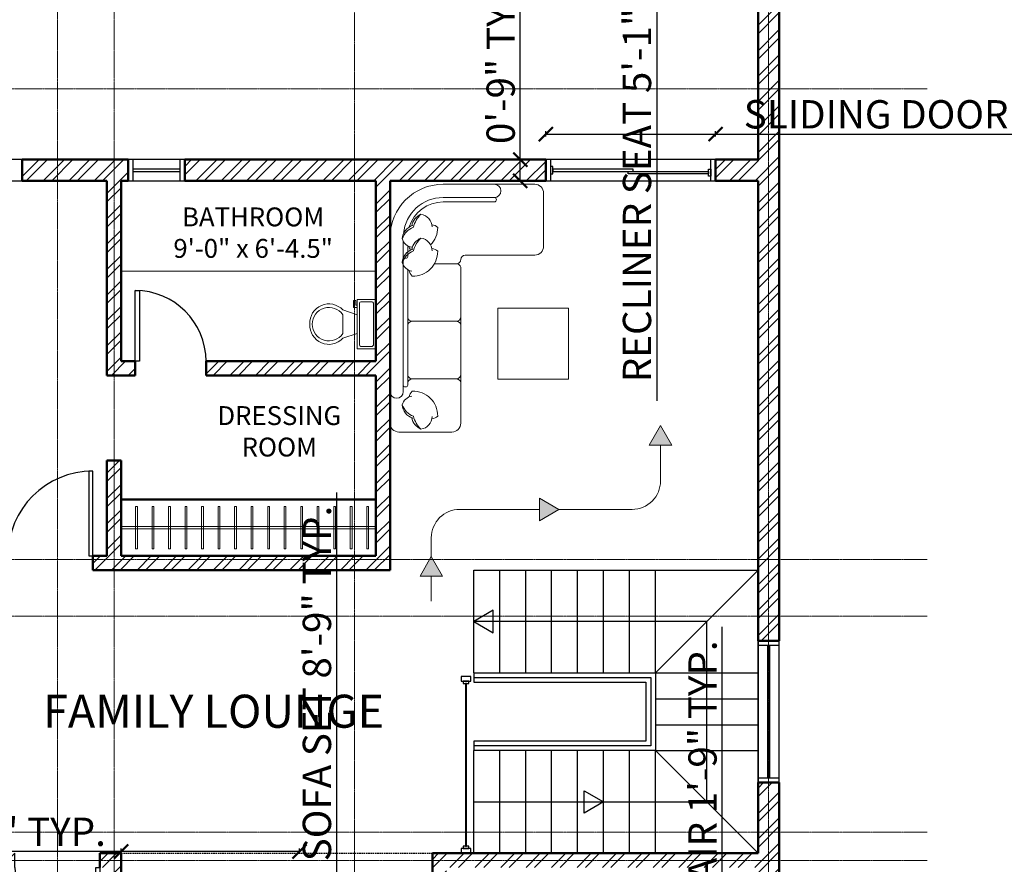
# Model space of a CAD drawing. Units: inches. Extents: x 261 to 2725, y 291 to 1454.
# Tile 24 of 35: x 1407 to 1824, y 675 to 1033. Entities that reach past the tile are written whole.
import ezdxf

# ---------------------------------------------------------------- set-up
doc = ezdxf.new("R2010")
doc.units = ezdxf.units.IN
doc.linetypes.add('CENTER', pattern=[2, 1.25, -0.25, 0.25, -0.25])
doc.linetypes.add('DASHED', pattern=[19.05, 12.7, -6.35])
for name, color, linetype, lineweight in [('A-ANNO-DIMS', 136, 'Continuous', 18), ('A-ANNO-SYMB', 7, 'Continuous', 18), ('A-AREA-IDEN', 18, 'Continuous', 18), ('A-DOOR', 160, 'Continuous', 25), ('A-FLOR-FIXT', 145, 'Continuous', 18), ('A-FLOR-HRAL', 132, 'Continuous', 25), ('A-FLOR-STRS', 42, 'Continuous', 25), ('A-FURN', 30, 'Continuous', 18), ('A-GLAZ', 150, 'Continuous', 25), ('A-GRID', 251, 'CENTER', 13), ('A-WALL', 222, 'Continuous', 50), ('A-WALL-OVHD', 222, 'DASHED', 25), ('A-WALL-PATT', 243, 'Continuous', 13)]:
    doc.layers.add(name, color=color, linetype=linetype, lineweight=lineweight)
doc.styles.get("Standard").update_dxf_attribs({"font": 'arial.ttf'})
doc.dimstyles.new('ISO-25', dxfattribs={"dimtxt": 12, "dimasz": 6, "dimexe": 1.25, "dimexo": 0.625, "dimtad": 1, "dimdec": 0, "dimlunit": 3, "dimtxsty": 'Standard', "dimblk": 'ARCHTICK', "dimcen": 2.5, "dimadec": 0, "dimazin": 0, "dimtfac": 1, "dimtdec": 0, "dimtmove": 0, "dimatfit": 3, "dimfxl": 1, "dimfxlon": 1, "dimarcsym": 0})

# ---------------------------------------------------------------- blocks, each defined once
blk = doc.blocks.new('*U6')
for p, q in [((-36, 0), (-36, 6)), ((0, 0), (0, 6))]:
    blk.add_line(p, q)
blk.add_lwpolyline([(0, 0), (0, -36), (-1.75, -36), (-1.75, 0)], close=True)
blk.add_arc((0, 0), 36, 180, 270)
blk = doc.blocks.new('*U7')
for p, q in [((0, 0), (0, -6)), ((-36, 0), (-36, -6))]:
    blk.add_line(p, q)
blk.add_lwpolyline([(0, 0), (0, 36), (-1.75, 36), (-1.75, 0)], close=True)
blk.add_arc((0, 0), 36, 90, 180)
blk = doc.blocks.new('*U8')
for p, q in [((0, 0), (0, -6)), ((30, 0), (30, -6))]:
    blk.add_line(p, q)
blk.add_lwpolyline([(0, 0), (0, 30), (1.75, 30), (1.75, 0)], close=True)
blk.add_arc((0, 0), 30, 0, 90)
blk = doc.blocks.new('A$C714C64AF')
for p, q in [((3108, 2017, -5499), (1005, 2017, -5499)), ((908, 1917, -5499), (908, 1317, -5499)), ((1365, 1867, -5499), (2793, 1867, -5499)), ((3508, 1417, -5499), (3508, 839, -5499)), ((3558, 1417, -5499), (3558, 839, -5499)), ((3708, 1417, -5499), (3708, 839, -5499)), ((1008, 1217, -5499), (1458, 1217, -5499)), ((1558, 1217, -5499), (1458, 1217, -5499)), ((1558, 1217, -5499), (2760, 1217, -5499)), ((2209, 1217, -5499), (2109, 1217, -5499)), ((2908, 1167, -5499), (2908, 381, -5499)), ((3708, 839, -5499), (3708, 381, -5499)), ((3008, 281, -5499), (3608, 281, -5499))]:
    blk.add_line(p, q)
at = {"elevation": -5499}
for points in [[(940, 1667, -0.14773), (1086, 1753, -0.213343), (1215, 1879)], [(1058, 1544, 0.165541), (1089, 1478, 0.425989), (1370, 1765, 0.121523), (1303, 1804)], [(1066, 1760, -0.306663), (1215, 1879, -0.30633), (1312, 1770)], [(1456, 1817), (1438, 1817, -0.414214), (1418, 1837), (1418, 1847, -0.414214), (1438, 1867)], [(1458, 1817, -0.414214), (1508, 1767)], [(1558, 1817, 0.414214), (1508, 1767), (1508, 1267, 0.432452)], [(1558, 1817, 0.414214), (1508, 1767)], [(2670, 1867), (1884, 1867, 0.414214)], [(2109, 1817, -0.414214), (2159, 1767)], [(2209, 1817, 0.414214), (2159, 1767), (2159, 1267, 0.432452)], [(2209, 1817, 0.414214), (2159, 1767)], [(2982, 1544, -0.165541), (2951, 1478, -0.425989), (2670, 1765, -0.121523), (2737, 1804)], [(2974, 1760, 0.306663), (2825, 1879, 0.30633), (2727, 1770)], [(3068, 1867), (2753, 1867, 0.415492)], [(3100, 1667, 0.14773), (2954, 1753, 0.213343), (2825, 1879)], [(3013, 1867), (2891, 1867, 0.414214), (2871, 1847), (2871, 1837, 0.414214), (2891, 1817), (2963, 1817, 0.414214)], [(2964, 1785, -0.071865), (3006, 1804)], [(3243, 1760, 0.306663), (3094, 1879, 0.30633), (2997, 1770)], [(3369, 1667, 0.14773), (3223, 1753, 0.213343), (3094, 1879)], [(1083, 1541, -0.356772), (940, 1667, -0.249542), (1070, 1771)], [(2957, 1541, 0.356772), (3100, 1667, 0.249542), (2970, 1771)], [(3226, 1541, 0.356772), (3369, 1667, 0.249542), (3239, 1771)], [(3251, 1544, -0.165541), (3220, 1478, -0.200231), (3022, 1559)]]:
    blk.add_lwpolyline(points, format="xyb", dxfattribs=at)
for points in [[(1458, 1817), (2743, 1817)], [(1884, 1867), (2670, 1867)], [(2944, 1817), (3012, 1817)], [(2810, 1515), (2810, 1267)]]:
    blk.add_lwpolyline(points, dxfattribs=at)
blk.add_lwpolyline([(2306, 800), (1506, 800), (1506, 0), (2306, 0)], close=True, dxfattribs=at)
for centre, radius, start, end in [((1008, 1917, -5499), 100, 90, 180), ((1365, 1942, -5499), 75, 90, 270), ((3108, 1417, -5499), 600, 0, 90), ((3108, 1417, -5499), 450, 0, 84.5853), ((3108, 1417, -5499), 400, 0, 72.9371), ((1008, 1317, -5499), 100, 180, 270), ((1458, 1267, -5499), 50, 270, 0), ((1458, 1267, -5499), 50, 270, 0), ((1558, 1267, -5499), 50, 180, 270), ((1558, 1267, -5499), 50, 180, 270), ((2109, 1267, -5499), 50, 270, 0), ((2109, 1267, -5499), 50, 270, 0), ((2209, 1267, -5499), 50, 180, 270), ((2209, 1267, -5499), 50, 180, 270), ((2760, 1267, -5499), 50, 270, 0), ((2760, 1267, -5499), 50, 270, 0), ((2860, 1267, -5499), 50, 180, 270), ((2860, 1267, -5499), 50, 180, 270), ((2858, 1167, -5499), 50, 0, 90), ((3533, 839, -5499), 25, 180, 0), ((3633, 839, -5499), 75, 180, 0), ((3008, 381, -5499), 100, 180, 270), ((3608, 381, -5499), 100, 270, 0)]:
    blk.add_arc(centre, radius, start, end)
blk = doc.blocks.new('*U27')
for p, q in [((9.5, -6), (9.5, -2)), ((-8, -8.5), (-8, -8)), ((-7, -8), (-7, -9.5)), ((-4, -8), (-6, -14)), ((4, -8), (6, -14)), ((-10, -8.5), (-8, -8.5)), ((-10, -9.5), (-10, -8.5)), ((-7, -9.5), (-10, -9.5)), ((4, -14), (-4, -14))]:
    blk.add_line(p, q)
blk.add_lwpolyline([(10.5, -8), (10.5, 0), (-10.5, 0), (-10.5, -8)], close=True)
for points in [[(-9.5, -2), (-9.5, -6)], [(8.5, -1), (-8.5, -1)], [(-8.5, -7), (8.5, -7)]]:
    blk.add_lwpolyline(points)
for centre, radius, start, end in [((-8.625, -1.875), 0.8839, 81.8699, 188.1301), ((8.625, -1.875), 0.8839, 351.8699, 98.1301), ((-8.625, -6.125), 0.8839, 171.869898, 278.1301), ((8.625, -6.125), 0.8839, 261.8699, 8.1301), ((-0.4772, -19.9188), 8.0953, 133.01722, 273.38), ((0.0374, -19.8731), 7.127, 124.50543, 269.7), ((-0.0373, -19.8731), 7.127, 270.3, 55.4946), ((0.4773, -19.9188), 8.0953, 266.62, 46.9828)]:
    blk.add_arc(centre, radius, start, end)
blk = doc.blocks.new('WIN-24')
for p, q in [((1455.08, 973.47), (1455.08, 964.47)), ((1475.08, 964.47), (1475.08, 973.47)), ((1475.08, 969.47), (1455.08, 969.47)), ((1455.08, 968.47), (1475.08, 968.47))]:
    blk.add_line(p, q)
blk.add_lwpolyline([(1477.08, 964.47), (1477.08, 973.47), (1453.08, 973.47), (1453.08, 964.47)], close=True)
blk = doc.blocks.new('DOOR-SLIDING-72')
for p, q in [((1632.08, 973.47), (1632.08, 964.47)), ((1700.08, 964.47), (1700.08, 973.47))]:
    blk.add_line(p, q)
for points in [[(1702.08, 964.47), (1702.08, 973.47), (1630.08, 973.47), (1630.08, 964.47)], [(1632.08, 967.47), (1633.08, 967.47), (1633.08, 970.47), (1632.08, 970.47)], [(1633.08, 968.47), (1667.08, 968.47), (1667.08, 969.47), (1633.08, 969.47)], [(1699.08, 967.47), (1665.08, 967.47), (1665.08, 968.47), (1699.08, 968.47)], [(1700.08, 966.47), (1699.08, 966.47), (1699.08, 969.47), (1700.08, 969.47)]]:
    blk.add_lwpolyline(points, close=True)
blk = doc.blocks.new('_ArchTick')
at = {"color": 0, "linetype": 'ByBlock', "const_width": 0.15}
blk.add_lwpolyline([(-0.5, -0.5), (0.5, 0.5)], dxfattribs=at)
blk = doc.blocks.new('*D37')
at = {"layer": 'A-ANNO-DIMS', "color": 0, "lineweight": -2, "ltscale": 0.07, "transparency": 16777216}
for p, q in [((1678.14, 1150), (1675.89, 1150)), ((1677.14, 1150), (1677.14, 1088.8)), ((1678.14, 1088.8), (1675.89, 1088.8)), ((1677.14, 1088.8), (1677.14, 871.16))]:
    blk.add_line(p, q, dxfattribs=at)
at = {"layer": 'Defpoints', "color": 0, "ltscale": 0.07, "transparency": 16777216}
for p in [(1686.32, 1150), (1677.14, 1088.8), (1686.32, 1088.8)]:
    blk.add_point(p, dxfattribs=at)
at = {"layer": 'A-ANNO-DIMS', "color": 0, "lineweight": -2, "ltscale": 0.07, "transparency": 16777216, "xscale": 6, "yscale": 6, "zscale": 6}
for p, rotation in [((1677.14, 1150), 90), ((1677.14, 1088.8), 270)]:
    blk.add_blockref('_ArchTick', p, dxfattribs=dict(at, rotation=rotation))
at = {"layer": 'A-ANNO-DIMS', "color": 0, "ltscale": 0.07, "transparency": 16777216, "insert": (1670.31, 976.98), "char_height": 12, "attachment_point": 5, "rotation": 90}
blk.add_mtext('RECLINER SEAT 5\'-1" TYP.', dxfattribs=at)
blk = doc.blocks.new('*D49')
at = {"layer": 'A-ANNO-DIMS', "color": 0, "lineweight": -2, "ltscale": 0.07, "transparency": 16777216}
for p, q in [((1704.93, 588.57), (1704.93, 775.49)), ((1703.93, 588.57), (1706.18, 588.57)), ((1704.93, 567.57), (1704.93, 588.57)), ((1703.93, 567.57), (1706.18, 567.57))]:
    blk.add_line(p, q, dxfattribs=at)
at = {"layer": 'Defpoints', "color": 0, "ltscale": 0.07, "transparency": 16777216}
for p in [(1701.78, 588.57), (1704.93, 588.57), (1701.78, 567.57)]:
    blk.add_point(p, dxfattribs=at)
at = {"layer": 'A-ANNO-DIMS', "color": 0, "lineweight": -2, "ltscale": 0.07, "transparency": 16777216, "xscale": 6, "yscale": 6, "zscale": 6}
for p, rotation in [((1704.93, 588.57), 90), ((1704.93, 567.57), 270)]:
    blk.add_blockref('_ArchTick', p, dxfattribs=dict(at, rotation=rotation))
at = {"layer": 'A-ANNO-DIMS', "color": 0, "ltscale": 0.07, "transparency": 16777216, "insert": (1698.1, 685.03), "char_height": 12, "attachment_point": 5, "rotation": 90}
blk.add_mtext('DESK CHAIR 1\'-9" TYP.', dxfattribs=at)
blk = doc.blocks.new('*D55')
at = {"layer": 'A-ANNO-DIMS', "color": 0, "lineweight": -2, "ltscale": 0.07, "transparency": 16777216}
for p, q in [((1541.46, 664.47), (1541.46, 832.37)), ((1540.46, 664.47), (1542.71, 664.47)), ((1541.46, 559.47), (1541.46, 664.47)), ((1540.46, 559.47), (1542.71, 559.47))]:
    blk.add_line(p, q, dxfattribs=at)
at = {"layer": 'Defpoints', "color": 0, "ltscale": 0.07, "transparency": 16777216}
for p in [(1525.71, 664.47), (1541.46, 664.47), (1525.71, 559.47)]:
    blk.add_point(p, dxfattribs=at)
at = {"layer": 'A-ANNO-DIMS', "color": 0, "lineweight": -2, "ltscale": 0.07, "transparency": 16777216, "xscale": 6, "yscale": 6, "zscale": 6}
for p, rotation in [((1541.46, 664.47), 90), ((1541.46, 559.47), 270)]:
    blk.add_blockref('_ArchTick', p, dxfattribs=dict(at, rotation=rotation))
at = {"layer": 'A-ANNO-DIMS', "color": 0, "ltscale": 0.07, "transparency": 16777216, "insert": (1534.63, 751.42), "char_height": 12, "attachment_point": 5, "rotation": 90}
blk.add_mtext('SOFA SET 8\'-9" TYP.', dxfattribs=at)
blk = doc.blocks.new('*D56')
at = {"layer": 'A-ANNO-DIMS', "color": 0, "lineweight": -2, "ltscale": 0.07, "transparency": 16777216}
for p, q in [((1450.08, 679.22), (1450.08, 681.47)), ((1525.71, 679.22), (1525.71, 681.47)), ((1450.08, 680.22), (1341.66, 680.22)), ((1525.71, 680.22), (1450.08, 680.22))]:
    blk.add_line(p, q, dxfattribs=at)
at = {"layer": 'Defpoints', "color": 0, "ltscale": 0.07, "transparency": 16777216}
for p in [(1450.08, 680.22), (1450.08, 664.47), (1525.71, 664.47)]:
    blk.add_point(p, dxfattribs=at)
at = {"layer": 'A-ANNO-DIMS', "color": 0, "lineweight": -2, "ltscale": 0.07, "transparency": 16777216, "xscale": 6, "yscale": 6, "zscale": 6, "rotation": 180}
blk.add_blockref('_ArchTick', (1450.08, 680.22), dxfattribs=at)
at = {"layer": 'A-ANNO-DIMS', "color": 0, "lineweight": -2, "ltscale": 0.07, "transparency": 16777216, "xscale": 6, "yscale": 6, "zscale": 6}
blk.add_blockref('_ArchTick', (1525.71, 680.22), dxfattribs=at)
at = {"layer": 'A-ANNO-DIMS', "color": 0, "ltscale": 0.07, "transparency": 16777216, "insert": (1392.87, 687.05), "char_height": 12, "attachment_point": 5}
blk.add_mtext('6\'-3 1/2" TYP.', dxfattribs=at)
blk = doc.blocks.new('*D63')
at = {"layer": 'A-ANNO-DIMS', "color": 0, "lineweight": -2, "ltscale": 0.07, "transparency": 16777216}
for p, q in [((1630.08, 983.27), (1630.08, 985.52)), ((1702.08, 983.27), (1702.08, 985.52)), ((1630.08, 984.27), (1702.08, 984.27)), ((1702.08, 984.27), (1909.1, 984.27))]:
    blk.add_line(p, q, dxfattribs=at)
at = {"layer": 'Defpoints', "color": 0, "ltscale": 0.07, "transparency": 16777216}
for p in [(1702.08, 984.27), (1630.08, 973.47), (1702.08, 973.47)]:
    blk.add_point(p, dxfattribs=at)
at = {"layer": 'A-ANNO-DIMS', "color": 0, "lineweight": -2, "ltscale": 0.07, "transparency": 16777216, "xscale": 6, "yscale": 6, "zscale": 6, "rotation": 180}
blk.add_blockref('_ArchTick', (1630.08, 984.27), dxfattribs=at)
at = {"layer": 'A-ANNO-DIMS', "color": 0, "lineweight": -2, "ltscale": 0.07, "transparency": 16777216, "xscale": 6, "yscale": 6, "zscale": 6}
blk.add_blockref('_ArchTick', (1702.08, 984.27), dxfattribs=at)
at = {"layer": 'A-ANNO-DIMS', "color": 0, "ltscale": 0.07, "transparency": 16777216, "insert": (1808.59, 991.1), "char_height": 12, "attachment_point": 5}
blk.add_mtext('SLIDING DOOR 6\'-0" TYP.', dxfattribs=at)
blk = doc.blocks.new('*D64')
at = {"layer": 'A-ANNO-DIMS', "color": 0, "lineweight": -2, "ltscale": 0.07, "transparency": 16777216}
for p, q in [((1619.28, 973.47), (1619.28, 1053.86)), ((1620.28, 973.47), (1618.03, 973.47)), ((1619.28, 964.47), (1619.28, 973.47)), ((1620.28, 964.47), (1618.03, 964.47))]:
    blk.add_line(p, q, dxfattribs=at)
at = {"layer": 'Defpoints', "color": 0, "ltscale": 0.07, "transparency": 16777216}
for p in [(1619.28, 973.47), (1630.08, 973.47), (1630.08, 964.47)]:
    blk.add_point(p, dxfattribs=at)
at = {"layer": 'A-ANNO-DIMS', "color": 0, "lineweight": -2, "ltscale": 0.07, "transparency": 16777216, "xscale": 6, "yscale": 6, "zscale": 6}
for p, rotation in [((1619.28, 973.47), 90), ((1619.28, 964.47), 270)]:
    blk.add_blockref('_ArchTick', p, dxfattribs=dict(at, rotation=rotation))
at = {"layer": 'A-ANNO-DIMS', "color": 0, "ltscale": 0.07, "transparency": 16777216, "insert": (1612.53, 1016.67), "char_height": 12, "attachment_point": 5, "rotation": 90}
blk.add_mtext('0\'-9" TYP.', dxfattribs=at)
blk = doc.blocks.new('*D82')
at = {"layer": 'A-ANNO-DIMS', "color": 0, "lineweight": -2, "ltscale": 0.07, "transparency": 16777216}
for p, q in [((2600.96, 679.47), (2603.21, 679.47)), ((2601.96, 517.47), (2601.96, 679.47)), ((2600.96, 517.47), (2603.21, 517.47))]:
    blk.add_line(p, q, dxfattribs=at)
at = {"layer": 'Defpoints', "color": 0, "ltscale": 0.07, "transparency": 16777216}
for p in [(946.45, 679.47), (2601.96, 679.47), (946.45, 517.47)]:
    blk.add_point(p, dxfattribs=at)
at = {"layer": 'A-ANNO-DIMS', "color": 0, "lineweight": -2, "ltscale": 0.07, "transparency": 16777216, "xscale": 6, "yscale": 6, "zscale": 6}
for p, rotation in [((2601.96, 679.47), 90), ((2601.96, 517.47), 270)]:
    blk.add_blockref('_ArchTick', p, dxfattribs=dict(at, rotation=rotation))
at = {"layer": 'A-ANNO-DIMS', "color": 0, "ltscale": 0.07, "transparency": 16777216, "insert": (2595.2, 598.47), "char_height": 12, "attachment_point": 5, "rotation": 90}
blk.add_mtext('13\'-6"', dxfattribs=at)
blk = doc.blocks.new('*D83')
at = {"layer": 'A-ANNO-DIMS', "color": 0, "lineweight": -2, "ltscale": 0.07, "transparency": 16777216}
for p, q in [((2600.96, 799.47), (2603.21, 799.47)), ((2601.96, 679.47), (2601.96, 799.47)), ((2600.96, 679.47), (2603.21, 679.47))]:
    blk.add_line(p, q, dxfattribs=at)
at = {"layer": 'Defpoints', "color": 0, "ltscale": 0.07, "transparency": 16777216}
for p in [(946.45, 799.47), (2601.96, 799.47), (946.45, 679.47)]:
    blk.add_point(p, dxfattribs=at)
at = {"layer": 'A-ANNO-DIMS', "color": 0, "lineweight": -2, "ltscale": 0.07, "transparency": 16777216, "xscale": 6, "yscale": 6, "zscale": 6}
for p, rotation in [((2601.96, 799.47), 90), ((2601.96, 679.47), 270)]:
    blk.add_blockref('_ArchTick', p, dxfattribs=dict(at, rotation=rotation))
at = {"layer": 'A-ANNO-DIMS', "color": 0, "ltscale": 0.07, "transparency": 16777216, "insert": (2595.21, 739.47), "char_height": 12, "attachment_point": 5, "rotation": 90}
blk.add_mtext('10\'-0"', dxfattribs=at)
blk = doc.blocks.new('*D84')
at = {"layer": 'A-ANNO-DIMS', "color": 0, "lineweight": -2, "ltscale": 0.07, "transparency": 16777216}
for p, q in [((2600.96, 1024.47), (2603.21, 1024.47)), ((2601.96, 799.47), (2601.96, 1024.47)), ((2600.96, 799.47), (2603.21, 799.47))]:
    blk.add_line(p, q, dxfattribs=at)
at = {"layer": 'Defpoints', "color": 0, "ltscale": 0.07, "transparency": 16777216}
for p in [(946.45, 1024.47), (2601.96, 1024.47), (946.45, 799.47)]:
    blk.add_point(p, dxfattribs=at)
at = {"layer": 'A-ANNO-DIMS', "color": 0, "lineweight": -2, "ltscale": 0.07, "transparency": 16777216, "xscale": 6, "yscale": 6, "zscale": 6}
for p, rotation in [((2601.96, 1024.47), 90), ((2601.96, 799.47), 270)]:
    blk.add_blockref('_ArchTick', p, dxfattribs=dict(at, rotation=rotation))
at = {"layer": 'A-ANNO-DIMS', "color": 0, "ltscale": 0.07, "transparency": 16777216, "insert": (2595.21, 911.97), "char_height": 12, "attachment_point": 5, "rotation": 90}
blk.add_mtext('18\'-9"', dxfattribs=at)
blk = doc.blocks.new('*D85')
at = {"layer": 'A-ANNO-DIMS', "color": 0, "lineweight": -2, "ltscale": 0.07, "transparency": 16777216}
for p, q in [((2600.96, 1222.47), (2603.21, 1222.47)), ((2601.96, 1024.47), (2601.96, 1222.47)), ((2600.96, 1024.47), (2603.21, 1024.47))]:
    blk.add_line(p, q, dxfattribs=at)
at = {"layer": 'Defpoints', "color": 0, "ltscale": 0.07, "transparency": 16777216}
for p in [(946.45, 1222.47), (2601.96, 1222.47), (946.45, 1024.47)]:
    blk.add_point(p, dxfattribs=at)
at = {"layer": 'A-ANNO-DIMS', "color": 0, "lineweight": -2, "ltscale": 0.07, "transparency": 16777216, "xscale": 6, "yscale": 6, "zscale": 6}
for p, rotation in [((2601.96, 1222.47), 90), ((2601.96, 1024.47), 270)]:
    blk.add_blockref('_ArchTick', p, dxfattribs=dict(at, rotation=rotation))
at = {"layer": 'A-ANNO-DIMS', "color": 0, "ltscale": 0.07, "transparency": 16777216, "insert": (2595.21, 1123.47), "char_height": 12, "attachment_point": 5, "rotation": 90}
blk.add_mtext('16\'-6"', dxfattribs=at)
blk = doc.blocks.new('*D112')
at = {"layer": 'A-ANNO-DIMS', "color": 0, "lineweight": -2, "ltscale": 0.07, "transparency": 16777216}
for p, q in [((2600.96, 679.47), (2603.21, 679.47)), ((2601.96, 550.47), (2601.96, 679.47)), ((2600.96, 550.47), (2603.21, 550.47))]:
    blk.add_line(p, q, dxfattribs=at)
at = {"layer": 'Defpoints', "color": 0, "ltscale": 0.07, "transparency": 16777216}
for p in [(1720.08, 679.47), (2601.96, 679.47), (1720.08, 550.47)]:
    blk.add_point(p, dxfattribs=at)
at = {"layer": 'A-ANNO-DIMS', "color": 0, "lineweight": -2, "ltscale": 0.07, "transparency": 16777216, "xscale": 6, "yscale": 6, "zscale": 6}
for p, rotation in [((2601.96, 679.47), 90), ((2601.96, 550.47), 270)]:
    blk.add_blockref('_ArchTick', p, dxfattribs=dict(at, rotation=rotation))
at = {"layer": 'A-ANNO-DIMS', "color": 0, "ltscale": 0.07, "transparency": 16777216, "insert": (2595.21, 614.97), "char_height": 12, "attachment_point": 5, "rotation": 90}
blk.add_mtext('10\'-9"', dxfattribs=at)
blk = doc.blocks.new('*D113')
at = {"layer": 'A-ANNO-DIMS', "color": 0, "lineweight": -2, "ltscale": 0.07, "transparency": 16777216}
for p, q in [((2600.96, 799.47), (2603.21, 799.47)), ((2601.96, 679.47), (2601.96, 799.47)), ((2600.96, 679.47), (2603.21, 679.47))]:
    blk.add_line(p, q, dxfattribs=at)
at = {"layer": 'Defpoints', "color": 0, "ltscale": 0.07, "transparency": 16777216}
for p in [(1720.08, 799.47), (2601.96, 799.47), (1720.08, 679.47)]:
    blk.add_point(p, dxfattribs=at)
at = {"layer": 'A-ANNO-DIMS', "color": 0, "lineweight": -2, "ltscale": 0.07, "transparency": 16777216, "xscale": 6, "yscale": 6, "zscale": 6}
for p, rotation in [((2601.96, 799.47), 90), ((2601.96, 679.47), 270)]:
    blk.add_blockref('_ArchTick', p, dxfattribs=dict(at, rotation=rotation))
at = {"layer": 'A-ANNO-DIMS', "color": 0, "ltscale": 0.07, "transparency": 16777216, "insert": (2595.21, 739.47), "char_height": 12, "attachment_point": 5, "rotation": 90}
blk.add_mtext('10\'-0"', dxfattribs=at)
blk = doc.blocks.new('*D114')
at = {"layer": 'A-ANNO-DIMS', "color": 0, "lineweight": -2, "ltscale": 0.07, "transparency": 16777216}
for p, q in [((2600.96, 964.47), (2603.21, 964.47)), ((2601.96, 799.47), (2601.96, 964.47)), ((2600.96, 799.47), (2603.21, 799.47))]:
    blk.add_line(p, q, dxfattribs=at)
at = {"layer": 'Defpoints', "color": 0, "ltscale": 0.07, "transparency": 16777216}
for p in [(1720.08, 964.47), (2601.96, 964.47), (1720.08, 799.47)]:
    blk.add_point(p, dxfattribs=at)
at = {"layer": 'A-ANNO-DIMS', "color": 0, "lineweight": -2, "ltscale": 0.07, "transparency": 16777216, "xscale": 6, "yscale": 6, "zscale": 6}
for p, rotation in [((2601.96, 964.47), 90), ((2601.96, 799.47), 270)]:
    blk.add_blockref('_ArchTick', p, dxfattribs=dict(at, rotation=rotation))
at = {"layer": 'A-ANNO-DIMS', "color": 0, "ltscale": 0.07, "transparency": 16777216, "insert": (2595.2, 881.97), "char_height": 12, "attachment_point": 5, "rotation": 90}
blk.add_mtext('13\'-9"', dxfattribs=at)
blk = doc.blocks.new('*D115')
at = {"layer": 'A-ANNO-DIMS', "color": 0, "lineweight": -2, "ltscale": 0.07, "transparency": 16777216}
for p, q in [((2600.96, 1222.47), (2603.21, 1222.47)), ((2601.96, 964.47), (2601.96, 1222.47)), ((2600.96, 964.47), (2603.21, 964.47))]:
    blk.add_line(p, q, dxfattribs=at)
at = {"layer": 'Defpoints', "color": 0, "ltscale": 0.07, "transparency": 16777216}
for p in [(1720.08, 1222.47), (2601.96, 1222.47), (1720.08, 964.47)]:
    blk.add_point(p, dxfattribs=at)
at = {"layer": 'A-ANNO-DIMS', "color": 0, "lineweight": -2, "ltscale": 0.07, "transparency": 16777216, "xscale": 6, "yscale": 6, "zscale": 6}
for p, rotation in [((2601.96, 1222.47), 90), ((2601.96, 964.47), 270)]:
    blk.add_blockref('_ArchTick', p, dxfattribs=dict(at, rotation=rotation))
at = {"layer": 'A-ANNO-DIMS', "color": 0, "ltscale": 0.07, "transparency": 16777216, "insert": (2595.21, 1093.47), "char_height": 12, "attachment_point": 5, "rotation": 90}
blk.add_mtext('21\'-6"', dxfattribs=at)
blk = doc.blocks.new('*D117')
at = {"layer": 'A-ANNO-DIMS', "color": 0, "lineweight": -2, "ltscale": 0.07, "transparency": 16777216}
for p, q in [((1588.08, 1437.76), (1588.08, 1440.01)), ((1702.08, 1437.76), (1702.08, 1440.01)), ((1588.08, 1438.76), (1702.08, 1438.76))]:
    blk.add_line(p, q, dxfattribs=at)
at = {"layer": 'Defpoints', "color": 0, "ltscale": 0.07, "transparency": 16777216}
for p in [(1702.08, 1438.76), (1588.08, 559.47), (1702.08, 559.47)]:
    blk.add_point(p, dxfattribs=at)
at = {"layer": 'A-ANNO-DIMS', "color": 0, "lineweight": -2, "ltscale": 0.07, "transparency": 16777216, "xscale": 6, "yscale": 6, "zscale": 6, "rotation": 180}
blk.add_blockref('_ArchTick', (1588.08, 1438.76), dxfattribs=at)
at = {"layer": 'A-ANNO-DIMS', "color": 0, "lineweight": -2, "ltscale": 0.07, "transparency": 16777216, "xscale": 6, "yscale": 6, "zscale": 6}
blk.add_blockref('_ArchTick', (1702.08, 1438.76), dxfattribs=at)
at = {"layer": 'A-ANNO-DIMS', "color": 0, "ltscale": 0.07, "transparency": 16777216, "insert": (1645.08, 1445.51), "char_height": 12, "attachment_point": 5}
blk.add_mtext('9\'-6"', dxfattribs=at)
blk = doc.blocks.new('*D120')
at = {"layer": 'A-ANNO-DIMS', "color": 0, "lineweight": -2, "ltscale": 0.07, "transparency": 16777216}
for p, q in [((2600.96, 880.73), (2603.21, 880.73)), ((2601.96, 805.47), (2601.96, 880.73)), ((2600.96, 805.47), (2603.21, 805.47))]:
    blk.add_line(p, q, dxfattribs=at)
at = {"layer": 'Defpoints', "color": 0, "ltscale": 0.07, "transparency": 16777216}
for p in [(1559.08, 880.73), (2601.96, 880.73), (1558.08, 805.47)]:
    blk.add_point(p, dxfattribs=at)
at = {"layer": 'A-ANNO-DIMS', "color": 0, "lineweight": -2, "ltscale": 0.07, "transparency": 16777216, "xscale": 6, "yscale": 6, "zscale": 6}
for p, rotation in [((2601.96, 880.73), 90), ((2601.96, 805.47), 270)]:
    blk.add_blockref('_ArchTick', p, dxfattribs=dict(at, rotation=rotation))
at = {"layer": 'A-ANNO-DIMS', "color": 0, "ltscale": 0.07, "transparency": 16777216, "insert": (2595.12, 843.1), "char_height": 12, "attachment_point": 5, "rotation": 90}
blk.add_mtext('6\'-3 1/2"', dxfattribs=at)
blk = doc.blocks.new('*D123')
at = {"layer": 'A-ANNO-DIMS', "color": 0, "lineweight": -2, "ltscale": 0.07, "transparency": 16777216}
for p, q in [((287.06, 1054.85), (284.81, 1054.85)), ((286.06, 439.47), (286.06, 1054.85)), ((287.06, 439.47), (284.81, 439.47))]:
    blk.add_line(p, q, dxfattribs=at)
at = {"layer": 'Defpoints', "color": 0, "ltscale": 0.07, "transparency": 16777216}
for p in [(286.06, 1054.85), (2007.71, 1054.85), (2007.71, 439.47)]:
    blk.add_point(p, dxfattribs=at)
at = {"layer": 'A-ANNO-DIMS', "color": 0, "lineweight": -2, "ltscale": 0.07, "transparency": 16777216, "xscale": 6, "yscale": 6, "zscale": 6}
for p, rotation in [((286.06, 1054.85), 90), ((286.06, 439.47), 270)]:
    blk.add_blockref('_ArchTick', p, dxfattribs=dict(at, rotation=rotation))
at = {"layer": 'A-ANNO-DIMS', "color": 0, "ltscale": 0.07, "transparency": 16777216, "insert": (279.22, 747.16), "char_height": 12, "attachment_point": 5, "rotation": 90}
blk.add_mtext('51\'-3 1/2"', dxfattribs=at)

msp = doc.modelspace()

# ---------------------------------------------------------------- hatches: boundary and pattern name
at = {"layer": 'A-ANNO-SYMB'}
h = msp.add_hatch(color=256, dxfattribs=at)
h.dxf.hatch_style = 1
h.paths.add_polyline_path([(1635.7, 825.23), (1627.39, 830.03), (1627.39, 820.43)])
h.paths.add_polyline_path([(1678.73, 860.77), (1673.94, 852.47), (1683.53, 852.47)])
h.paths.add_polyline_path([(1581.58, 805.28), (1576.78, 796.98), (1586.37, 796.98)])
h.paths.add_polyline_path([(724.45, 497.71), (717.86, 490.1), (731.04, 490.1)])
h.paths.add_polyline_path([(724.45, 506.59), (717.86, 498.98), (731.04, 498.98)])
at = {"layer": 'A-WALL-PATT'}
h = msp.add_hatch(dxfattribs=at)
h.set_pattern_fill('ANSI32', color=256, scale=0.8)
h.paths.add_polyline_path([(478.45, 685.47), (580.45, 685.47), (580.45, 691.47), (577.45, 691.47), (577.45, 694.47), (571.45, 694.47), (571.45, 691.47), (478.45, 691.47), (478.45, 721.47), (469.45, 721.47), (469.45, 508.47), (538.45, 508.47), (538.45, 517.47), (478.45, 517.47)])
h.paths.add_polyline_path([(694.45, 517.47), (676.45, 517.47), (676.45, 646.47), (670.45, 646.47), (670.45, 517.47), (610.45, 517.47), (610.45, 508.47), (694.45, 508.47)])
h.paths.add_polyline_path([(676.45, 784.47), (478.45, 784.47), (478.45, 844.47), (469.45, 844.47), (469.45, 745.47), (478.45, 745.47), (478.45, 775.47), (571.45, 775.47), (571.45, 724.47), (577.45, 724.47), (577.45, 775.47), (670.45, 775.47), (670.45, 691.47), (610.45, 691.47), (610.45, 685.47), (670.45, 685.47), (670.45, 682.47), (676.45, 682.47)])
h.paths.add_polyline_path([(955.45, 880.47), (946.45, 880.47), (946.45, 808.47), (778.45, 808.47), (778.45, 799.47), (946.45, 799.47), (946.45, 517.47), (898.45, 517.47), (898.45, 508.47), (955.45, 508.47)])
h.paths.add_polyline_path([(778.45, 598.47), (772.45, 598.47), (772.45, 517.47), (754.45, 517.47), (754.45, 508.47), (826.45, 508.47), (826.45, 517.47), (778.45, 517.47)])
h.paths.add_polyline_path([(955.45, 1090.47), (946.45, 1090.47), (946.45, 1030.47), (817.45, 1030.47), (817.45, 1024.47), (946.45, 1024.47), (946.45, 952.47), (955.45, 952.47)])
h.paths.add_polyline_path([(955.45, 1231.47), (730.45, 1231.47), (730.45, 1222.47), (772.45, 1222.47), (772.45, 1096.47), (766.45, 1096.47), (766.45, 1090.47), (772.45, 1090.47), (772.45, 1006.47), (712.45, 1006.47), (712.45, 1000.47), (778.45, 1000.47), (778.45, 1024.47), (781.45, 1024.47), (781.45, 1030.47), (778.45, 1030.47), (778.45, 1222.47), (946.45, 1222.47), (946.45, 1162.47), (955.45, 1162.47)])
h.paths.add_polyline_path([(694.45, 1231.47), (619.45, 1231.47), (619.45, 1222.47), (646.45, 1222.47), (646.45, 1039.47), (652.45, 1039.47), (652.45, 1090.47), (736.45, 1090.47), (736.45, 1096.47), (652.45, 1096.47), (652.45, 1222.47), (694.45, 1222.47)])
h.paths.add_polyline_path([(571.45, 1231.47), (469.45, 1231.47), (469.45, 1099.47), (478.45, 1099.47), (478.45, 1144.47), (544.45, 1144.47), (544.45, 1153.47), (538.45, 1153.47), (538.45, 1150.47), (478.45, 1150.47), (478.45, 1222.47), (538.45, 1222.47), (538.45, 1183.47), (544.45, 1183.47), (544.45, 1222.47), (571.45, 1222.47)])
h.paths.add_polyline_path([(538.45, 1006.47), (478.45, 1006.47), (478.45, 1051.47), (469.45, 1051.47), (469.45, 940.47), (478.45, 940.47), (478.45, 1000.47), (538.45, 1000.47)])
h.paths.add_polyline_path([(652.45, 1006.47), (652.45, 1009.47), (646.45, 1009.47), (646.45, 1006.47), (586.45, 1006.47), (586.45, 1000.47), (652.45, 1000.47)])
h.paths.add_polyline_path([(1288.08, 973.47), (1243.08, 973.47), (1243.08, 920.97), (1252.08, 920.97), (1252.08, 964.47), (1288.08, 964.47)], flags=17)
h.paths.add_polyline_path([(1402.08, 805.47), (1252.08, 805.47), (1252.08, 848.97), (1243.08, 848.97), (1243.08, 757.47), (1252.08, 757.47), (1252.08, 799.47), (1294.08, 799.47), (1372.08, 799.47), (1372.08, 779.47), (1372.08, 715.47), (1378.08, 715.47), (1378.08, 799.47), (1402.08, 799.47)])
h.paths.add_polyline_path([(1252.08, 721.47), (1243.08, 721.47), (1243.08, 439.47), (1729.08, 439.47), (1729.08, 709.47), (1720.08, 709.47), (1720.08, 679.47), (1582.08, 679.47), (1582.08, 670.47), (1588.08, 670.47), (1588.08, 673.47), (1720.08, 673.47), (1720.08, 559.47), (1690.08, 559.47), (1690.08, 550.47), (1720.08, 550.47), (1720.08, 448.47), (1252.08, 448.47), (1252.08, 496.47), (1312.08, 496.47), (1312.08, 505.47), (1252.08, 505.47), (1252.08, 673.47), (1405.08, 673.47), (1405.08, 679.47), (1378.08, 679.47), (1378.08, 685.47), (1372.08, 685.47), (1372.08, 679.47), (1252.08, 679.47)])
h.paths.add_polyline_path([(1450.08, 550.47), (1480.08, 550.47), (1480.08, 559.47), (1450.08, 559.47), (1450.08, 679.47), (1441.08, 679.47), (1441.08, 673.47), (1444.08, 673.47), (1444.08, 505.47), (1384.08, 505.47), (1384.08, 496.47), (1450.08, 496.47)], flags=17)
h.paths.add_polyline_path([(1618.08, 559.47), (1588.08, 559.47), (1588.08, 634.47), (1582.08, 634.47), (1582.08, 559.47), (1552.08, 559.47), (1552.08, 550.47), (1618.08, 550.47)], flags=17)
h.paths.add_polyline_path([(1564.08, 964.47), (1630.08, 964.47), (1630.08, 973.47), (1477.08, 973.47), (1477.08, 964.47), (1558.08, 964.47), (1558.08, 926.22), (1558.08, 887.97), (1486.08, 887.97), (1486.08, 881.97), (1558.08, 881.97), (1558.08, 805.47), (1450.08, 805.47), (1450.08, 845.97), (1444.08, 845.97), (1444.08, 805.47), (1438.08, 805.47), (1438.08, 799.47), (1564.08, 799.47)], flags=17)
h.paths.add_polyline_path([(1453.08, 973.47), (1408.08, 973.47), (1408.08, 964.47), (1444.08, 964.47), (1444.08, 881.97), (1450.08, 881.97), (1456.08, 881.97), (1456.08, 887.97), (1450.08, 887.97), (1450.08, 964.47), (1453.08, 964.47)], flags=17)
h.paths.add_polyline_path([(1729.08, 1231.47), (1243.08, 1231.47), (1243.08, 1167.47), (1252.08, 1167.47), (1252.08, 1222.47), (1441.08, 1222.47), (1441.08, 1045.47), (1648.08, 1045.47), (1648.08, 1051.47), (1450.08, 1051.47), (1450.08, 1074.47), (1450.08, 1222.47), (1472.08, 1222.47), (1720.08, 1222.47), (1720.08, 1051.47), (1708.08, 1051.47), (1708.08, 1045.47), (1720.08, 1045.47), (1720.08, 973.47), (1702.08, 973.47), (1702.08, 964.47), (1720.08, 964.47), (1720.08, 769.47), (1729.08, 769.47)])
h.paths.add_polyline_path([(2493.71, 1054.85), (2007.71, 1054.85), (2007.71, 439.47), (2214.67, 439.47), (2214.67, 496.47), (2493.71, 496.47)])
h.paths.add_polyline_path([(2016.71, 1045.85), (2304.71, 1045.85), (2304.71, 841.47), (2310.71, 841.47), (2310.71, 1045.85), (2484.71, 1045.85), (2484.71, 805.47), (2310.71, 805.47), (2310.71, 811.47), (2304.71, 811.47), (2304.71, 799.47), (2484.71, 799.47), (2484.71, 679.47), (2304.71, 679.47), (2304.71, 673.47), (2484.71, 673.47), (2484.71, 505.47), (2208.67, 505.47), (2208.67, 448.47), (2016.71, 448.47), (2016.71, 799.47), (2304.71, 799.47), (2304.71, 805.47), (2016.71, 805.47)], flags=16)

# ---------------------------------------------------------------- linework, layer by layer
at = {"layer": 'A-ANNO-SYMB', "ltscale": 0.03}
msp.add_line((1581.58, 786.26), (1581.58, 796.98), dxfattribs=at)
at = {"layer": 'A-ANNO-SYMB'}
for points in [[(1678.73, 860.77), (1673.94, 852.47), (1683.53, 852.47)], [(1635.7, 825.23), (1627.39, 830.03), (1627.39, 820.43)], [(1581.58, 805.28), (1576.78, 796.98), (1586.37, 796.98)]]:
    msp.add_lwpolyline(points, close=True, dxfattribs=at)
at = {"layer": 'A-ANNO-SYMB', "ltscale": 0.03}
for points in [[(1635.7, 825.23), (1666.73, 825.23, 0.414214), (1678.73, 837.23), (1678.73, 852.47)], [(1627.39, 825.23), (1593.58, 825.23, 0.414214), (1581.58, 813.23), (1581.58, 805.28)]]:
    msp.add_lwpolyline(points, format="xyb", dxfattribs=at)
at = {"layer": 'A-DOOR'}
msp.add_lwpolyline([(1408.08, 964.47), (1408.08, 973.47), (1288.08, 973.47), (1288.08, 964.47)], close=True, dxfattribs=at)
at = {"layer": 'A-FLOR-FIXT'}
msp.add_lwpolyline([(1450.08, 964.47), (1558.08, 964.47), (1558.08, 926.22), (1450.08, 926.22)], close=True, dxfattribs=at)
at = {"layer": 'A-FLOR-HRAL'}
for points in [[(1594.28, 752.44), (1598.28, 752.44), (1598.28, 754.44), (1594.28, 754.44)], [(1595.03, 751.44), (1597.53, 751.44), (1597.53, 752.44), (1595.03, 752.44)], [(1596.03, 682.47), (1596.53, 682.47), (1596.53, 751.44), (1596.03, 751.44)], [(1594.28, 679.47), (1598.28, 679.47), (1598.28, 681.47), (1594.28, 681.47)], [(1595.03, 681.47), (1597.53, 681.47), (1597.53, 682.47), (1595.03, 682.47)]]:
    msp.add_lwpolyline(points, close=True, dxfattribs=at)
at = {"layer": 'A-FLOR-STRS', "ltscale": 0.2}
for p, q in [((1599.58, 755.97), (1599.58, 799.47)), ((1599.58, 799.47), (1720.08, 799.47)), ((1610.58, 755.97), (1610.58, 799.47)), ((1621.58, 755.97), (1621.58, 799.47)), ((1632.58, 755.97), (1632.58, 799.47)), ((1643.58, 755.97), (1643.58, 799.47)), ((1654.58, 755.97), (1654.58, 799.47)), ((1665.58, 755.97), (1665.58, 799.47)), ((1676.58, 755.97), (1676.58, 799.47)), ((1676.58, 755.97), (1720.08, 799.47)), ((1720.08, 679.47), (1720.08, 799.47)), ((1698.33, 777.72), (1599.58, 777.72)), ((1698.33, 701.22), (1698.33, 777.72)), ((1599.58, 755.97), (1599.58, 751.97)), ((1676.58, 755.97), (1720.08, 755.97)), ((1676.58, 744.97), (1720.08, 744.97)), ((1676.58, 733.97), (1720.08, 733.97)), ((1599.58, 726.97), (1599.58, 722.97)), ((1599.58, 679.47), (1599.58, 722.97)), ((1610.58, 679.47), (1610.58, 722.97)), ((1621.58, 679.47), (1621.58, 722.97)), ((1632.58, 679.47), (1632.58, 722.97)), ((1643.58, 679.47), (1643.58, 722.97)), ((1654.58, 679.47), (1654.58, 722.97)), ((1665.58, 679.47), (1665.58, 722.97)), ((1676.58, 722.97), (1720.08, 722.97)), ((1676.58, 679.47), (1676.58, 722.97)), ((1676.58, 722.97), (1720.08, 679.47)), ((1599.58, 701.22), (1698.33, 701.22)), ((1599.58, 679.47), (1720.08, 679.47))]:
    msp.add_line(p, q, dxfattribs=at)
for points in [[(1599.58, 777.72), (1607.83, 772.96), (1607.83, 782.48)], [(1654.58, 701.22), (1646.33, 696.46), (1646.33, 705.98)]]:
    msp.add_lwpolyline(points, close=True, dxfattribs=at)
for points in [[(1599.58, 755.97), (1676.58, 755.97), (1676.58, 722.97), (1599.58, 722.97)], [(1599.58, 753.97), (1674.58, 753.97), (1674.58, 724.97), (1599.58, 724.97)], [(1599.58, 751.97), (1672.58, 751.97), (1672.58, 726.97), (1599.58, 726.97)]]:
    msp.add_lwpolyline(points, dxfattribs=at)
at = {"layer": 'A-FURN'}
for p, q in [((1558.08, 817.97), (1450.08, 817.97)), ((1558.08, 816.97), (1450.08, 816.97))]:
    msp.add_line(p, q, dxfattribs=at)
for points in [[(1456.2, 826.47), (1456.2, 808.47), (1456.95, 808.47), (1456.95, 826.47)], [(1463.2, 826.47), (1463.2, 808.47), (1463.95, 808.47), (1463.95, 826.47)], [(1470.2, 826.47), (1470.2, 808.47), (1470.95, 808.47), (1470.95, 826.47)], [(1477.2, 826.47), (1477.2, 808.47), (1477.95, 808.47), (1477.95, 826.47)], [(1484.2, 826.47), (1484.2, 808.47), (1484.95, 808.47), (1484.95, 826.47)], [(1491.2, 826.47), (1491.2, 808.47), (1491.95, 808.47), (1491.95, 826.47)], [(1498.2, 826.47), (1498.2, 808.47), (1498.95, 808.47), (1498.95, 826.47)], [(1505.2, 826.47), (1505.2, 808.47), (1505.95, 808.47), (1505.95, 826.47)], [(1512.2, 826.47), (1512.2, 808.47), (1512.95, 808.47), (1512.95, 826.47)], [(1519.2, 826.47), (1519.2, 808.47), (1519.95, 808.47), (1519.95, 826.47)], [(1526.2, 826.47), (1526.2, 808.47), (1526.95, 808.47), (1526.95, 826.47)], [(1533.2, 826.47), (1533.2, 808.47), (1533.95, 808.47), (1533.95, 826.47)], [(1540.2, 826.47), (1540.2, 808.47), (1540.95, 808.47), (1540.95, 826.47)], [(1547.2, 826.47), (1547.2, 808.47), (1547.95, 808.47), (1547.95, 826.47)], [(1554.2, 826.47), (1554.2, 808.47), (1554.95, 808.47), (1554.95, 826.47)]]:
    msp.add_lwpolyline(points, close=True, dxfattribs=at)
at = {"layer": 'A-GLAZ'}
for p, q in [((1729.08, 767.47), (1720.08, 767.47)), ((1724.08, 767.47), (1724.08, 711.47)), ((1725.08, 711.47), (1725.08, 767.47)), ((1720.08, 711.47), (1729.08, 711.47))]:
    msp.add_line(p, q, dxfattribs=at)
msp.add_lwpolyline([(1729.08, 709.47), (1729.08, 769.47), (1720.08, 769.47), (1720.08, 709.47)], close=True, dxfattribs=at)
at = {"layer": 'A-GRID', "ltscale": 0.5}
for p, q in [((1423.08, 1330.51), (1423.08, 416.51)), ((1447.08, 1330.51), (1447.08, 416.51)), ((1549.08, 1330.47), (1549.08, 416.47)), ((1724.58, 1330.47), (1724.58, 416.47)), ((1167.93, 1003.47), (1791.93, 1003.47)), ((1167.93, 803.97), (1791.93, 803.97)), ((1167.93, 779.97), (1791.93, 779.97)), ((1167.93, 688.47), (1791.93, 688.47)), ((1167.93, 676.47), (1791.93, 676.47))]:
    msp.add_line(p, q, dxfattribs=at)
at = {"layer": 'A-WALL'}
for p, q in [((1729.08, 1231.47), (1729.08, 769.47)), ((1720.08, 1045.47), (1720.08, 973.47)), ((1408.08, 964.47), (1408.08, 973.47)), ((1453.08, 973.47), (1408.08, 973.47)), ((1453.08, 964.47), (1453.08, 973.47)), ((1477.08, 964.47), (1477.08, 973.47)), ((1630.08, 973.47), (1477.08, 973.47)), ((1630.08, 964.47), (1630.08, 973.47)), ((1720.08, 973.47), (1702.08, 973.47)), ((1702.08, 964.47), (1702.08, 973.47)), ((1444.08, 964.47), (1408.08, 964.47)), ((1444.08, 964.47), (1444.08, 881.97)), ((1450.08, 964.47), (1450.08, 887.97)), ((1453.08, 964.47), (1450.08, 964.47)), ((1558.08, 964.47), (1477.08, 964.47)), ((1558.08, 964.47), (1558.08, 887.97)), ((1564.08, 964.47), (1564.08, 799.47)), ((1630.08, 964.47), (1564.08, 964.47)), ((1720.08, 964.47), (1702.08, 964.47)), ((1720.08, 964.47), (1720.08, 769.47)), ((1456.08, 887.97), (1450.08, 887.97)), ((1456.08, 881.97), (1456.08, 887.97)), ((1558.08, 887.97), (1486.08, 887.97)), ((1486.08, 881.97), (1486.08, 887.97)), ((1450.08, 881.97), (1444.08, 881.97)), ((1456.08, 881.97), (1450.08, 881.97)), ((1558.08, 881.97), (1486.08, 881.97)), ((1558.08, 881.97), (1558.08, 805.47)), ((1450.08, 845.97), (1444.08, 845.97)), ((1444.08, 845.97), (1444.08, 805.47)), ((1450.08, 845.97), (1450.08, 805.47)), ((1450.08, 829.47), (1558.08, 829.47)), ((1438.08, 805.47), (1438.08, 799.47)), ((1438.08, 805.47), (1444.08, 805.47)), ((1450.08, 805.47), (1558.08, 805.47)), ((1438.08, 799.47), (1564.08, 799.47)), ((1720.08, 769.47), (1729.08, 769.47)), ((1720.08, 709.47), (1729.08, 709.47)), ((1720.08, 709.47), (1720.08, 679.47)), ((1729.08, 709.47), (1729.08, 439.47)), ((1441.08, 673.47), (1441.08, 679.47)), ((1441.08, 679.47), (1450.08, 679.47)), ((1450.08, 559.47), (1450.08, 679.47)), ((1582.08, 679.47), (1720.08, 679.47)), ((1582.08, 670.47), (1582.08, 679.47))]:
    msp.add_line(p, q, dxfattribs=at)
at = {"layer": 'A-WALL-OVHD', "ltscale": 0.05}
msp.add_line((1450.08, 679.47), (1582.08, 679.47), dxfattribs=at)

# ---------------------------------------------------------------- block references
at = {"layer": 'A-DOOR'}
for name, p in [('DOOR-SLIDING-72', (0, 0)), ('*U8', (1456.08, 887.97)), ('*U7', (1438.08, 805.47)), ('*U6', (1441.08, 673.47))]:
    msp.add_blockref(name, p, dxfattribs=at)
at = {"layer": 'A-FLOR-FIXT', "rotation": 270.0002079578469}
msp.add_blockref('*U27', (1558.08, 903.73), dxfattribs=at)
at = {"layer": 'A-FURN', "xscale": 0.0375, "yscale": 0.0375, "zscale": 0.0375, "rotation": 90.00000000000003}
msp.add_blockref('A$C714C64AF', (1639.71, 823.96, 206.2), dxfattribs=at)
at = {"layer": 'A-GLAZ'}
msp.add_blockref('WIN-24', (0, 0), dxfattribs=at)

# ---------------------------------------------------------------- texts
at = {"layer": 'A-AREA-IDEN', "attachment_point": 1}
for s, width, insert, char_height in [('\\pxqc;{\\fTimes New Roman|b0|i0|c0|p18;BATHROOM\\P9\'-0" x 6\'-4.5"}', 72.1712, (1469.96, 953.17), 8), ('\\pxqc;{\\fTimes New Roman|b0|i0|c0|p18;DRESSING ROOM}', 72.1712, (1481.05, 868.97), 8), ('\\pxqc;{\\fTimes New Roman|b0|i0|c0|p18;\\T1.25;FAMILY LOUNGE}', 215.629, (1381.44, 746.68), 14)]:
    msp.add_mtext_dynamic_manual_height_columns(s, width=width, gutter_width=12.5, heights=[0], dxfattribs=dict(at, insert=insert, char_height=char_height))

# ---------------------------------------------------------------- dimensions: what is measured, and where the dimension line sits
at = {"layer": 'A-ANNO-DIMS', "ltscale": 0.07}
dim = msp.add_linear_dim(base=(1702.08, 1438.76), p1=(1588.08, 559.47), p2=(1702.08, 559.47), dimstyle='ISO-25', override={"dimdec": 1, "dimlfac": 1, "dimrnd": 0, "dimzin": 1, "dimdsep": 46, "dimlunit": 4, "dimfrac": 2}, dxfattribs=at)
dim.commit()
dim.dimension.update_dxf_attribs({"geometry": '*D117', "text_midpoint": (1645.08, 1445.51)})
for base, p1, p2, picture, middle in [((2601.96, 1222.47), (946.45, 1024.47), (946.45, 1222.47), '*D85', (2595.21, 1123.47)), ((2601.96, 1222.47), (1720.08, 964.47), (1720.08, 1222.47), '*D115', (2595.21, 1093.47)), ((286.06, 1054.85), (2007.71, 439.47), (2007.71, 1054.85), '*D123', (279.22, 747.16)), ((2601.96, 1024.47), (946.45, 799.47), (946.45, 1024.47), '*D84', (2595.21, 911.97)), ((2601.96, 964.47), (1720.08, 799.47), (1720.08, 964.47), '*D114', (2595.2, 881.97)), ((2601.96, 880.73), (1558.08, 805.47), (1559.08, 880.73), '*D120', (2595.12, 843.1)), ((2601.96, 799.47), (946.45, 679.47), (946.45, 799.47), '*D83', (2595.21, 739.47)), ((2601.96, 799.47), (1720.08, 679.47), (1720.08, 799.47), '*D113', (2595.21, 739.47)), ((2601.96, 679.47), (946.45, 517.47), (946.45, 679.47), '*D82', (2595.2, 598.47)), ((2601.96, 679.47), (1720.08, 550.47), (1720.08, 679.47), '*D112', (2595.21, 614.97))]:
    dim = msp.add_linear_dim(base=base, p1=p1, p2=p2, angle=90, dimstyle='ISO-25', override={"dimdec": 1, "dimlfac": 1, "dimrnd": 0, "dimzin": 1, "dimdsep": 46, "dimlunit": 4, "dimfrac": 2}, dxfattribs=at)
    dim.commit()
    dim.dimension.update_dxf_attribs({"geometry": picture, "text_midpoint": middle})
for base, p1, p2, angle, text, picture, middle in [((1677.14, 1088.8), (1686.32, 1150), (1686.32, 1088.8), 270, 'RECLINER SEAT <> TYP.', '*D37', (1670.31, 976.98)), ((1619.28, 973.47), (1630.08, 964.47), (1630.08, 973.47), 90, '<> TYP.', '*D64', (1612.53, 1016.67)), ((1541.46, 664.47), (1525.71, 559.47), (1525.71, 664.47), 90, 'SOFA SET <> TYP.', '*D55', (1534.63, 751.42)), ((1704.93, 588.57), (1701.78, 567.57), (1701.78, 588.57), 90, 'DESK CHAIR <> TYP.', '*D49', (1698.1, 685.03)), ((1450.08, 680.22), (1525.71, 664.47), (1450.08, 664.47), 180, '<> TYP.', '*D56', (1392.87, 687.05))]:
    dim = msp.add_linear_dim(base=base, p1=p1, p2=p2, angle=angle, text=text, dimstyle='ISO-25', override={"dimdec": 1, "dimrnd": 0, "dimzin": 1, "dimlunit": 4, "dimfrac": 2}, dxfattribs=at)
    dim.commit()
    dim.dimension.update_dxf_attribs({"geometry": picture, "text_midpoint": middle})
dim = msp.add_linear_dim(base=(1702.08, 984.27), p1=(1630.08, 973.47), p2=(1702.08, 973.47), text='SLIDING DOOR <> TYP.', dimstyle='ISO-25', override={"dimdec": 1, "dimrnd": 0, "dimzin": 1, "dimlunit": 4, "dimfrac": 2}, dxfattribs=at)
dim.commit()
dim.dimension.update_dxf_attribs({"geometry": '*D63', "text_midpoint": (1808.59, 991.1)})

doc.saveas('drawing.dxf')
